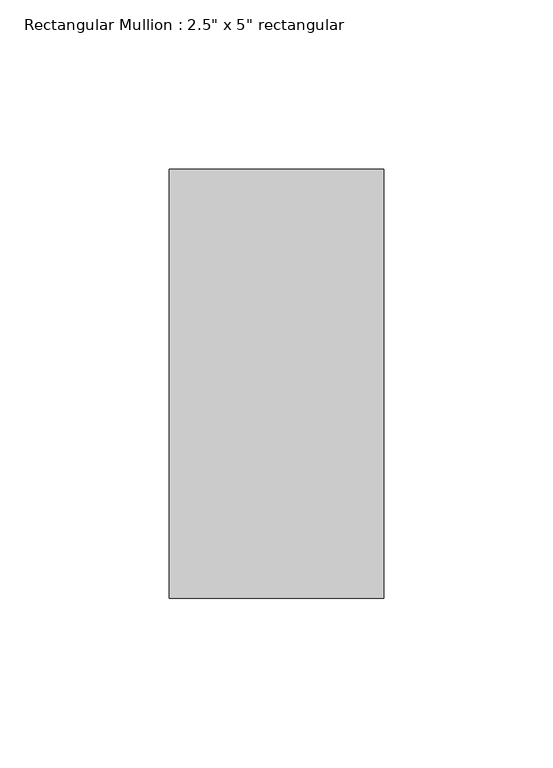
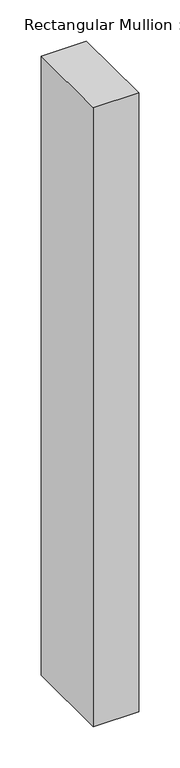
"""IFC4 building model written with IfcOpenShell, lengths in millimetres: member geometry."""

from ifc_helpers import new_model, si_unit, frame, origin, place, context, project, spatial, polyline, outline, extrude, source, transform, mapped, element, save


def member_d959a85f(model_context):
    return source(origin(), model_context, "Body", "SweptSolid", [
        extrude(outline(polyline([(0.0, 63.5), (0.0, -63.5), (-63.5, -63.5), (-63.5, 63.5), (0.0, 63.5)])), frame((0.0, 0.0, -918.7415583), z_axis=(0.0, 0.0, 1.0), x_axis=(1.0, 0.0, 0.0)), (0.0, 0.0, 1.0), 918.7415583),
    ])


if __name__ == "__main__":
    model = new_model("IFC4")
    model_context = context("Model", 3, world=origin())
    ifc_project = project(units=[si_unit("LENGTHUNIT", "METRE", prefix="MILLI")], contexts=[model_context])
    site = spatial("IfcSite", under=ifc_project)
    building = spatial("IfcBuilding", under=site)
    placement = place(None, origin())
    member_shape = member_d959a85f(model_context)
    element("IfcMember", 1, ObjectType="Rectangular Mullion : 2.5\" x 5\" rectangular", at=placement, inside=building, context=model_context, shape_type="MappedRepresentation", body=[
        mapped(member_shape, transform((0.0, 0.0, 0.0), x_axis=(1.0, 0.0, 0.0), y_axis=(0.0, 1.0, 0.0), z_axis=(0.0, 0.0, 1.0))),
    ])
    save(model, "model.ifc")

# Revit data of these elements
# Type "Rectangular Mullion : 2.5\" x 5\" rectangular"
#   built-in parameter 1007304 = 0.416667 (stored number, unit not read)
#   built-in parameter 1007301 = 0.104167 (stored number, unit not read)
#   built-in parameter 1007300 = 0.104167 (stored number, unit not read)
# Element 1 (IfcMember, "Rectangular Mullion : 2.5\" x 5\" rectangular")
#   Materials on its faces: "Aluminum"
# Materials
#   "Aluminum": class "Metal", colour RGB 247 247 247, transparency 0, Description = "Aluminum 6061", Cost = 0
